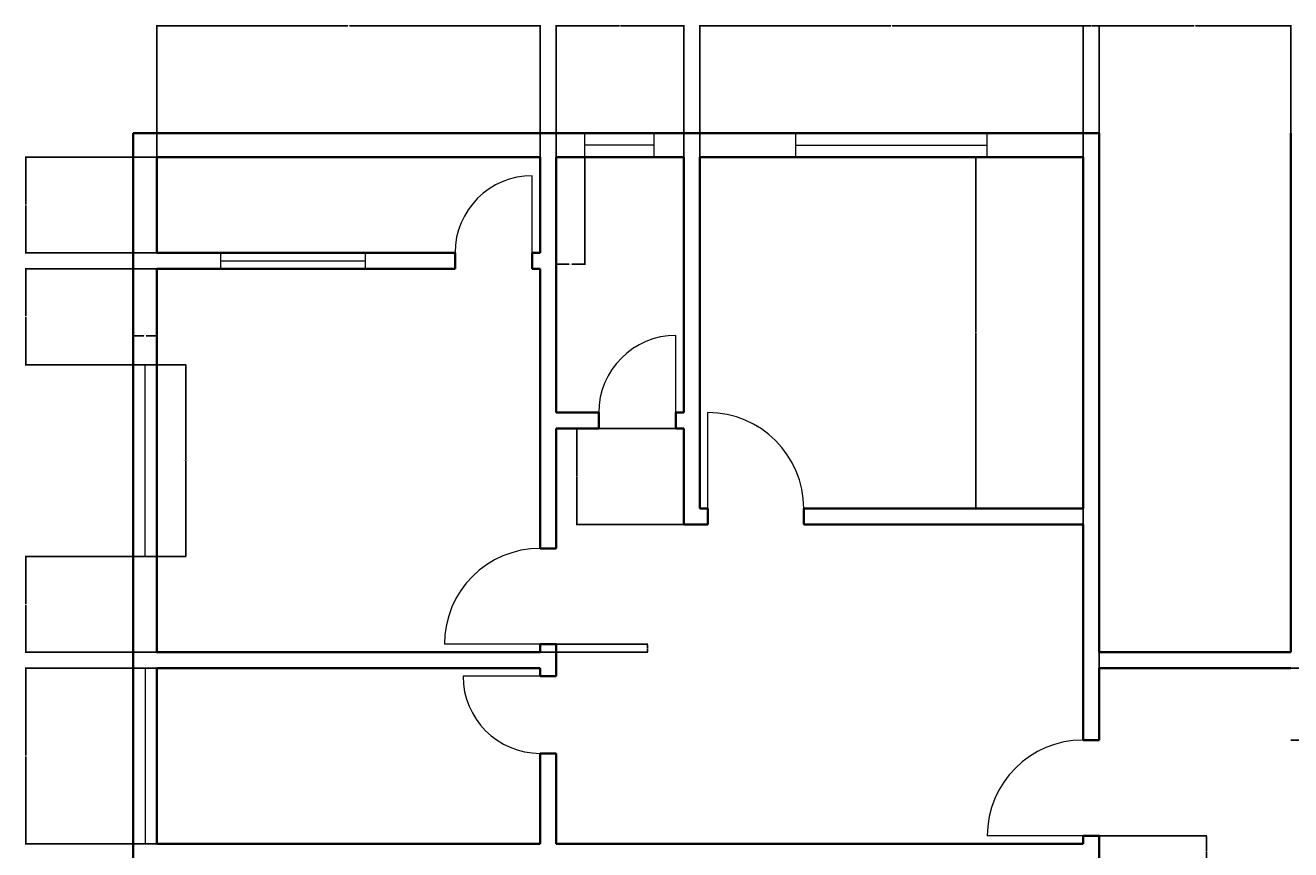
# Model space of a CAD drawing. Units: inches. Extents: x 2811 to 3694, y 2039 to 2670.
# Tile 2 of 3: x 2811 to 3286, y 2361 to 2670. Entities that reach past the tile are written whole.
import ezdxf

# ---------------------------------------------------------------- set-up
doc = ezdxf.new("R2010")
doc.units = ezdxf.units.IN
for name, color, linetype, lineweight in [('A-ANNO-DIMS', 2, 'Continuous', 18), ('A-DOOR', 3, 'Continuous', 18), ('A-GLAZ', 4, 'Continuous', 18), ('A-WALL', 7, 'Continuous', 35)]:
    doc.layers.add(name, color=color, linetype=linetype, lineweight=lineweight)
doc.styles.get("Standard").update_dxf_attribs({"font": 'arial.ttf'})
doc.dimstyles.get("Standard").update_dxf_attribs({"dimtxt": 0.18, "dimasz": 0.18, "dimexe": 0.18, "dimexo": 0.0625, "dimgap": 0.09, "dimtad": 0, "dimtih": 1, "dimtoh": 1, "dimdec": 4, "dimzin": 0, "dimdsep": 46, "dimtxsty": 'Standard', "dimcen": 0.09, "dimadec": 0, "dimazin": 0, "dimtfac": 1, "dimtdec": 4, "dimtofl": 0, "dimtmove": 0, "dimatfit": 3, "dimfxl": 1, "dimtolj": 1, "dimtzin": 0, "dimarcsym": 0})

# ---------------------------------------------------------------- blocks, each defined once
blk = doc.blocks.new('DOOR-SWING-29IN')
blk.add_line((29, 0), (29, 29))
blk.add_arc((29, 0), 29, 90, 180)
blk = doc.blocks.new('DOOR-SWING-36IN')
blk.add_line((36, 0), (0, 0))
blk.add_arc((36, 0), 36, 90, 180)
blk = doc.blocks.new('WIN-72IN')
for p, q in [((0, 0), (0, 9)), ((72, 0), (72, 9)), ((0, 4.5), (72, 4.5))]:
    blk.add_line(p, q)
blk = doc.blocks.new('WIN-66IN')
for p, q in [((0, 66), (9, 66)), ((4.5, 0), (4.5, 66)), ((0, 0), (9, 0))]:
    blk.add_line(p, q)
blk = doc.blocks.new('WIN-26_08IN')
for p, q in [((0, 0), (0, 9)), ((26.08, 0), (26.08, 9)), ((26.08, 4.5), (0, 4.5))]:
    blk.add_line(p, q)
blk = doc.blocks.new('*D14')
at = {"layer": 'A-ANNO-DIMS', "color": 0, "lineweight": -2, "transparency": 16777216}
for p, q in [((2860.34, 2542.98), (2871.26, 2542.98)), ((2871.08, 2542.8), (2871.08, 2507.16)), ((2871.08, 2471.16), (2871.08, 2506.8)), ((2860.34, 2470.98), (2871.26, 2470.98))]:
    blk.add_line(p, q, dxfattribs=at)
at = {"layer": 'A-ANNO-DIMS', "color": 0, "transparency": 16777216}
for points in [[(2871.05, 2542.8), (2871.11, 2542.8), (2871.08, 2542.98)], [(2871.05, 2471.16), (2871.11, 2471.16), (2871.08, 2470.98)]]:
    blk.add_solid(points, dxfattribs=at)
at = {"layer": 'Defpoints', "color": 0, "transparency": 16777216}
for p in [(2860.28, 2542.98), (2871.08, 2542.98), (2860.28, 2470.98)]:
    blk.add_point(p, dxfattribs=at)
at = {"layer": 'A-ANNO-DIMS', "color": 0, "transparency": 16777216, "insert": (2871.08, 2506.98), "char_height": 0.18, "attachment_point": 5}
blk.add_mtext('\\A1;WINDOW 72 TYP.', dxfattribs=at)
blk = doc.blocks.new('*D15')
at = {"layer": 'A-ANNO-DIMS', "color": 0, "lineweight": -2, "transparency": 16777216}
for p, q in [((2851.28, 2543.04), (2851.28, 2553.96)), ((2851.46, 2553.78), (2855.32, 2553.78)), ((2860.1, 2553.78), (2856.23, 2553.78)), ((2860.28, 2543.04), (2860.28, 2553.96))]:
    blk.add_line(p, q, dxfattribs=at)
at = {"layer": 'A-ANNO-DIMS', "color": 0, "transparency": 16777216}
for points in [[(2851.46, 2553.81), (2851.46, 2553.75), (2851.28, 2553.78)], [(2860.1, 2553.81), (2860.1, 2553.75), (2860.28, 2553.78)]]:
    blk.add_solid(points, dxfattribs=at)
at = {"layer": 'Defpoints', "color": 0, "transparency": 16777216}
for p in [(2851.28, 2553.78), (2851.28, 2542.98), (2860.28, 2542.98)]:
    blk.add_point(p, dxfattribs=at)
at = {"layer": 'A-ANNO-DIMS', "color": 0, "transparency": 16777216, "insert": (2855.78, 2553.78), "char_height": 0.18, "attachment_point": 5}
blk.add_mtext('\\A1;9 TYP.', dxfattribs=at)
blk = doc.blocks.new('*D24')
at = {"layer": 'A-ANNO-DIMS', "color": 0, "lineweight": -2, "transparency": 16777216}
for p, q in [((2860.28, 2621.04), (2860.28, 2670.46)), ((2860.46, 2670.28), (2932, 2670.28)), ((3004.1, 2670.28), (2932.56, 2670.28)), ((3004.28, 2621.04), (3004.28, 2670.46))]:
    blk.add_line(p, q, dxfattribs=at)
at = {"layer": 'A-ANNO-DIMS', "color": 0, "transparency": 16777216}
for points in [[(2860.46, 2670.31), (2860.46, 2670.25), (2860.28, 2670.28)], [(3004.1, 2670.31), (3004.1, 2670.25), (3004.28, 2670.28)]]:
    blk.add_solid(points, dxfattribs=at)
at = {"layer": 'Defpoints', "color": 0, "transparency": 16777216}
for p in [(3004.28, 2670.28), (2860.28, 2620.98), (3004.28, 2620.98)]:
    blk.add_point(p, dxfattribs=at)
at = {"layer": 'A-ANNO-DIMS', "color": 0, "transparency": 16777216, "insert": (2932.28, 2670.28), "char_height": 0.18, "attachment_point": 5}
blk.add_mtext('\\A1;144', dxfattribs=at)
blk = doc.blocks.new('*D25')
at = {"layer": 'A-ANNO-DIMS', "color": 0, "lineweight": -2, "transparency": 16777216}
for p, q in [((3010.28, 2621.04), (3010.28, 2670.46)), ((3010.46, 2670.28), (3034.05, 2670.28)), ((3058.1, 2670.28), (3034.5, 2670.28)), ((3058.28, 2621.04), (3058.28, 2670.46))]:
    blk.add_line(p, q, dxfattribs=at)
at = {"layer": 'A-ANNO-DIMS', "color": 0, "transparency": 16777216}
for points in [[(3010.46, 2670.31), (3010.46, 2670.25), (3010.28, 2670.28)], [(3058.1, 2670.31), (3058.1, 2670.25), (3058.28, 2670.28)]]:
    blk.add_solid(points, dxfattribs=at)
at = {"layer": 'Defpoints', "color": 0, "transparency": 16777216}
for p in [(3058.28, 2670.28), (3010.28, 2620.98), (3058.28, 2620.98)]:
    blk.add_point(p, dxfattribs=at)
at = {"layer": 'A-ANNO-DIMS', "color": 0, "transparency": 16777216, "insert": (3034.28, 2670.28), "char_height": 0.18, "attachment_point": 5}
blk.add_mtext('\\A1;48', dxfattribs=at)
blk = doc.blocks.new('*D26')
at = {"layer": 'A-ANNO-DIMS', "color": 0, "lineweight": -2, "transparency": 16777216}
for p, q in [((3064.28, 2621.04), (3064.28, 2670.46)), ((3064.46, 2670.28), (3136, 2670.28)), ((3208.1, 2670.28), (3136.56, 2670.28)), ((3208.28, 2621.04), (3208.28, 2670.46))]:
    blk.add_line(p, q, dxfattribs=at)
at = {"layer": 'A-ANNO-DIMS', "color": 0, "transparency": 16777216}
for points in [[(3064.46, 2670.31), (3064.46, 2670.25), (3064.28, 2670.28)], [(3208.1, 2670.31), (3208.1, 2670.25), (3208.28, 2670.28)]]:
    blk.add_solid(points, dxfattribs=at)
at = {"layer": 'Defpoints', "color": 0, "transparency": 16777216}
for p in [(3208.28, 2670.28), (3064.28, 2620.98), (3208.28, 2620.98)]:
    blk.add_point(p, dxfattribs=at)
at = {"layer": 'A-ANNO-DIMS', "color": 0, "transparency": 16777216, "insert": (3136.28, 2670.28), "char_height": 0.18, "attachment_point": 5}
blk.add_mtext('\\A1;144', dxfattribs=at)
blk = doc.blocks.new('*D27')
at = {"layer": 'A-ANNO-DIMS', "color": 0, "lineweight": -2, "transparency": 16777216}
for p, q in [((3214.28, 2630.04), (3214.28, 2670.46)), ((3214.46, 2670.28), (3250.06, 2670.28)), ((3286.1, 2670.28), (3250.49, 2670.28)), ((3286.28, 2630.04), (3286.28, 2670.46))]:
    blk.add_line(p, q, dxfattribs=at)
at = {"layer": 'A-ANNO-DIMS', "color": 0, "transparency": 16777216}
for points in [[(3214.46, 2670.31), (3214.46, 2670.25), (3214.28, 2670.28)], [(3286.1, 2670.31), (3286.1, 2670.25), (3286.28, 2670.28)]]:
    blk.add_solid(points, dxfattribs=at)
at = {"layer": 'Defpoints', "color": 0, "transparency": 16777216}
for p in [(3286.28, 2670.28), (3214.28, 2629.98), (3286.28, 2629.98)]:
    blk.add_point(p, dxfattribs=at)
at = {"layer": 'A-ANNO-DIMS', "color": 0, "transparency": 16777216, "insert": (3250.28, 2670.28), "char_height": 0.18, "attachment_point": 5}
blk.add_mtext('\\A1;72', dxfattribs=at)
blk = doc.blocks.new('*D31')
at = {"layer": 'A-ANNO-DIMS', "color": 0, "lineweight": -2, "transparency": 16777216}
for p, q in [((2860.21, 2620.98), (2810.8, 2620.98)), ((2810.98, 2620.8), (2810.98, 2603.16)), ((2810.98, 2585.16), (2810.98, 2602.8)), ((2860.21, 2584.98), (2810.8, 2584.98))]:
    blk.add_line(p, q, dxfattribs=at)
at = {"layer": 'A-ANNO-DIMS', "color": 0, "transparency": 16777216}
for points in [[(2810.95, 2620.8), (2811.01, 2620.8), (2810.98, 2620.98)], [(2810.95, 2585.16), (2811.01, 2585.16), (2810.98, 2584.98)]]:
    blk.add_solid(points, dxfattribs=at)
at = {"layer": 'Defpoints', "color": 0, "transparency": 16777216}
for p in [(2860.28, 2620.98), (2810.98, 2584.98), (2860.28, 2584.98)]:
    blk.add_point(p, dxfattribs=at)
at = {"layer": 'A-ANNO-DIMS', "color": 0, "transparency": 16777216, "insert": (2810.98, 2602.98), "char_height": 0.18, "attachment_point": 5}
blk.add_mtext('\\A1;36', dxfattribs=at)
blk = doc.blocks.new('*D32')
at = {"layer": 'A-ANNO-DIMS', "color": 0, "lineweight": -2, "transparency": 16777216}
for p, q in [((2860.21, 2578.98), (2810.8, 2578.98)), ((2810.98, 2578.8), (2810.98, 2561.16)), ((2810.98, 2543.16), (2810.98, 2560.8)), ((2860.21, 2542.98), (2810.8, 2542.98))]:
    blk.add_line(p, q, dxfattribs=at)
at = {"layer": 'A-ANNO-DIMS', "color": 0, "transparency": 16777216}
for points in [[(2810.95, 2578.8), (2811.01, 2578.8), (2810.98, 2578.98)], [(2810.95, 2543.16), (2811.01, 2543.16), (2810.98, 2542.98)]]:
    blk.add_solid(points, dxfattribs=at)
at = {"layer": 'Defpoints', "color": 0, "transparency": 16777216}
for p in [(2860.28, 2578.98), (2810.98, 2542.98), (2860.28, 2542.98)]:
    blk.add_point(p, dxfattribs=at)
at = {"layer": 'A-ANNO-DIMS', "color": 0, "transparency": 16777216, "insert": (2810.98, 2560.98), "char_height": 0.18, "attachment_point": 5}
blk.add_mtext('\\A1;36', dxfattribs=at)
blk = doc.blocks.new('*D33')
at = {"layer": 'A-ANNO-DIMS', "color": 0, "lineweight": -2, "transparency": 16777216}
for p, q in [((2860.21, 2470.98), (2810.8, 2470.98)), ((2810.98, 2470.8), (2810.98, 2453.16)), ((2810.98, 2435.16), (2810.98, 2452.8)), ((2860.21, 2434.98), (2810.8, 2434.98))]:
    blk.add_line(p, q, dxfattribs=at)
at = {"layer": 'A-ANNO-DIMS', "color": 0, "transparency": 16777216}
for points in [[(2810.95, 2470.8), (2811.01, 2470.8), (2810.98, 2470.98)], [(2810.95, 2435.16), (2811.01, 2435.16), (2810.98, 2434.98)]]:
    blk.add_solid(points, dxfattribs=at)
at = {"layer": 'Defpoints', "color": 0, "transparency": 16777216}
for p in [(2860.28, 2470.98), (2810.98, 2434.98), (2860.28, 2434.98)]:
    blk.add_point(p, dxfattribs=at)
at = {"layer": 'A-ANNO-DIMS', "color": 0, "transparency": 16777216, "insert": (2810.98, 2452.98), "char_height": 0.18, "attachment_point": 5}
blk.add_mtext('\\A1;36', dxfattribs=at)
blk = doc.blocks.new('*D34')
at = {"layer": 'A-ANNO-DIMS', "color": 0, "lineweight": -2, "transparency": 16777216}
for p, q in [((2860.21, 2428.98), (2810.8, 2428.98)), ((2810.98, 2428.8), (2810.98, 2396.16)), ((2810.98, 2363.16), (2810.98, 2395.8)), ((2860.21, 2362.98), (2810.8, 2362.98))]:
    blk.add_line(p, q, dxfattribs=at)
at = {"layer": 'A-ANNO-DIMS', "color": 0, "transparency": 16777216}
for points in [[(2810.95, 2428.8), (2811.01, 2428.8), (2810.98, 2428.98)], [(2810.95, 2363.16), (2811.01, 2363.16), (2810.98, 2362.98)]]:
    blk.add_solid(points, dxfattribs=at)
at = {"layer": 'Defpoints', "color": 0, "transparency": 16777216}
for p in [(2860.28, 2428.98), (2810.98, 2362.98), (2860.28, 2362.98)]:
    blk.add_point(p, dxfattribs=at)
at = {"layer": 'A-ANNO-DIMS', "color": 0, "transparency": 16777216, "insert": (2810.98, 2395.98), "char_height": 0.18, "attachment_point": 5}
blk.add_mtext('\\A1;66', dxfattribs=at)
blk = doc.blocks.new('*D40')
at = {"layer": 'A-ANNO-DIMS', "color": 0, "lineweight": -2, "transparency": 16777216}
for p, q in [((3058.21, 2518.98), (3017.8, 2518.98)), ((3017.98, 2518.8), (3017.98, 2501.16)), ((3017.98, 2483.16), (3017.98, 2500.8)), ((3058.21, 2482.98), (3017.8, 2482.98))]:
    blk.add_line(p, q, dxfattribs=at)
at = {"layer": 'A-ANNO-DIMS', "color": 0, "transparency": 16777216}
for points in [[(3017.95, 2518.8), (3018.01, 2518.8), (3017.98, 2518.98)], [(3017.95, 2483.16), (3018.01, 2483.16), (3017.98, 2482.98)]]:
    blk.add_solid(points, dxfattribs=at)
at = {"layer": 'Defpoints', "color": 0, "transparency": 16777216}
for p in [(3017.98, 2518.98), (3058.28, 2518.98), (3058.28, 2482.98)]:
    blk.add_point(p, dxfattribs=at)
at = {"layer": 'A-ANNO-DIMS', "color": 0, "transparency": 16777216, "insert": (3017.98, 2500.98), "char_height": 0.18, "attachment_point": 5}
blk.add_mtext('\\A1;36', dxfattribs=at)
blk = doc.blocks.new('*D41')
at = {"layer": 'A-ANNO-DIMS', "color": 0, "lineweight": -2, "transparency": 16777216}
for p, q in [((3208.21, 2620.98), (3167.8, 2620.98)), ((3167.98, 2620.8), (3167.98, 2555.16)), ((3167.98, 2489.16), (3167.98, 2554.8)), ((3208.21, 2488.98), (3167.8, 2488.98))]:
    blk.add_line(p, q, dxfattribs=at)
at = {"layer": 'A-ANNO-DIMS', "color": 0, "transparency": 16777216}
for points in [[(3167.95, 2620.8), (3168.01, 2620.8), (3167.98, 2620.98)], [(3167.95, 2489.16), (3168.01, 2489.16), (3167.98, 2488.98)]]:
    blk.add_solid(points, dxfattribs=at)
at = {"layer": 'Defpoints', "color": 0, "transparency": 16777216}
for p in [(3167.98, 2620.98), (3208.28, 2620.98), (3208.28, 2488.98)]:
    blk.add_point(p, dxfattribs=at)
at = {"layer": 'A-ANNO-DIMS', "color": 0, "transparency": 16777216, "insert": (3167.98, 2554.98), "char_height": 0.18, "attachment_point": 5}
blk.add_mtext('\\A1;132', dxfattribs=at)
blk = doc.blocks.new('*D52')
at = {"layer": 'A-ANNO-DIMS', "color": 0, "lineweight": -2, "transparency": 16777216}
for p, q in [((3010.28, 2620.92), (3010.28, 2580.5)), ((3021.03, 2620.92), (3021.03, 2580.5)), ((3010.46, 2580.68), (3015.2, 2580.68)), ((3020.85, 2580.68), (3016.11, 2580.68))]:
    blk.add_line(p, q, dxfattribs=at)
at = {"layer": 'A-ANNO-DIMS', "color": 0, "transparency": 16777216}
for points in [[(3010.46, 2580.71), (3010.46, 2580.65), (3010.28, 2580.68)], [(3020.85, 2580.71), (3020.85, 2580.65), (3021.03, 2580.68)]]:
    blk.add_solid(points, dxfattribs=at)
at = {"layer": 'Defpoints', "color": 0, "transparency": 16777216}
for p in [(3010.28, 2620.98), (3021.03, 2620.98), (3010.28, 2580.68)]:
    blk.add_point(p, dxfattribs=at)
at = {"layer": 'A-ANNO-DIMS', "color": 0, "transparency": 16777216, "insert": (3015.65, 2580.68), "char_height": 0.18, "attachment_point": 5}
blk.add_mtext('\\A1;10.754', dxfattribs=at)
blk = doc.blocks.new('*D54')
at = {"layer": 'A-ANNO-DIMS', "color": 0, "lineweight": -2, "transparency": 16777216}
for p, q in [((3004.34, 2437.98), (3044.76, 2437.98)), ((3004.34, 2434.98), (3044.76, 2434.98)), ((3044.58, 2437.8), (3044.58, 2436.66)), ((3044.58, 2435.16), (3044.58, 2436.3))]:
    blk.add_line(p, q, dxfattribs=at)
at = {"layer": 'A-ANNO-DIMS', "color": 0, "transparency": 16777216}
for points in [[(3044.55, 2437.8), (3044.61, 2437.8), (3044.58, 2437.98)], [(3044.55, 2435.16), (3044.61, 2435.16), (3044.58, 2434.98)]]:
    blk.add_solid(points, dxfattribs=at)
at = {"layer": 'Defpoints', "color": 0, "transparency": 16777216}
for p in [(3004.28, 2437.98), (3004.28, 2434.98), (3044.58, 2434.98)]:
    blk.add_point(p, dxfattribs=at)
at = {"layer": 'A-ANNO-DIMS', "color": 0, "transparency": 16777216, "insert": (3044.58, 2436.48), "char_height": 0.18, "attachment_point": 5}
blk.add_mtext('\\A1;3', dxfattribs=at)
blk = doc.blocks.new('*D60')
at = {"layer": 'A-ANNO-DIMS', "color": 0, "lineweight": -2, "transparency": 16777216}
for p, q in [((3286.34, 2428.98), (3326.76, 2428.98)), ((3326.58, 2428.8), (3326.58, 2415.66)), ((3326.58, 2402.16), (3326.58, 2415.3)), ((3286.34, 2401.98), (3326.76, 2401.98))]:
    blk.add_line(p, q, dxfattribs=at)
at = {"layer": 'A-ANNO-DIMS', "color": 0, "transparency": 16777216}
for points in [[(3326.55, 2428.8), (3326.61, 2428.8), (3326.58, 2428.98)], [(3326.55, 2402.16), (3326.61, 2402.16), (3326.58, 2401.98)]]:
    blk.add_solid(points, dxfattribs=at)
at = {"layer": 'Defpoints', "color": 0, "transparency": 16777216}
for p in [(3286.28, 2428.98), (3286.28, 2401.98), (3326.58, 2401.98)]:
    blk.add_point(p, dxfattribs=at)
at = {"layer": 'A-ANNO-DIMS', "color": 0, "transparency": 16777216, "insert": (3326.58, 2415.48), "char_height": 0.18, "attachment_point": 5}
blk.add_mtext('\\A1;27', dxfattribs=at)
blk = doc.blocks.new('*D61')
at = {"layer": 'A-ANNO-DIMS', "color": 0, "lineweight": -2, "transparency": 16777216}
for p, q in [((3208.28, 2402.04), (3208.28, 2670.46)), ((3208.46, 2670.28), (3211.13, 2670.28)), ((3214.1, 2670.28), (3211.43, 2670.28)), ((3214.28, 2402.04), (3214.28, 2670.46))]:
    blk.add_line(p, q, dxfattribs=at)
at = {"layer": 'A-ANNO-DIMS', "color": 0, "transparency": 16777216}
for points in [[(3208.46, 2670.31), (3208.46, 2670.25), (3208.28, 2670.28)], [(3214.1, 2670.31), (3214.1, 2670.25), (3214.28, 2670.28)]]:
    blk.add_solid(points, dxfattribs=at)
at = {"layer": 'Defpoints', "color": 0, "transparency": 16777216}
for p in [(3214.28, 2670.28), (3208.28, 2401.98), (3214.28, 2401.98)]:
    blk.add_point(p, dxfattribs=at)
at = {"layer": 'A-ANNO-DIMS', "color": 0, "transparency": 16777216, "insert": (3211.28, 2670.28), "char_height": 0.18, "attachment_point": 5}
blk.add_mtext('\\A1;6', dxfattribs=at)
blk = doc.blocks.new('*D62')
at = {"layer": 'A-ANNO-DIMS', "color": 0, "lineweight": -2, "transparency": 16777216}
for p, q in [((3214.34, 2365.98), (3254.76, 2365.98)), ((3254.58, 2365.8), (3254.58, 2360.16)), ((3254.58, 2354.16), (3254.58, 2359.8)), ((3214.34, 2353.98), (3254.76, 2353.98))]:
    blk.add_line(p, q, dxfattribs=at)
at = {"layer": 'A-ANNO-DIMS', "color": 0, "transparency": 16777216}
for points in [[(3254.55, 2365.8), (3254.61, 2365.8), (3254.58, 2365.98)], [(3254.55, 2354.16), (3254.61, 2354.16), (3254.58, 2353.98)]]:
    blk.add_solid(points, dxfattribs=at)
at = {"layer": 'Defpoints', "color": 0, "transparency": 16777216}
for p in [(3214.28, 2365.98), (3214.28, 2353.98), (3254.58, 2353.98)]:
    blk.add_point(p, dxfattribs=at)
at = {"layer": 'A-ANNO-DIMS', "color": 0, "transparency": 16777216, "insert": (3254.58, 2359.98), "char_height": 0.18, "attachment_point": 5}
blk.add_mtext('\\A1;12', dxfattribs=at)

msp = doc.modelspace()

# ---------------------------------------------------------------- linework, layer by layer
at = {"layer": 'A-GLAZ'}
for p, q in [((3100.2765, 2625.4792), (3172.2765, 2625.4792)), ((2884.2647, 2578.9792), (2884.2647, 2584.9792)), ((2884.2647, 2581.9792), (2938.6787, 2581.9792)), ((2884.2647, 2581.9792), (2938.6787, 2581.9792)), ((2938.6787, 2578.9792), (2938.6787, 2584.9792)), ((2851.2765, 2470.9792), (2851.2765, 2542.9792)), ((2860.2765, 2542.9792), (2855.7765, 2542.9792)), ((2851.2765, 2362.9792), (2851.2765, 2428.9792)), ((2860.2765, 2428.9792), (2855.7765, 2428.9792))]:
    msp.add_line(p, q, dxfattribs=at)
at = {"layer": 'A-WALL'}
for p, q in [((2851.2765, 2629.9792), (2851.2765, 2124.9792)), ((3214.2765, 2629.9792), (2851.2765, 2629.9792)), ((3214.2765, 2620.9792), (3214.2765, 2629.9792)), ((3286.2765, 2620.9792), (3286.2765, 2629.9792)), ((2860.2765, 2620.9792), (2860.2765, 2584.9792)), ((3004.2765, 2620.9792), (2860.2765, 2620.9792)), ((3004.2765, 2620.9792), (3004.2765, 2584.9792)), ((3010.2765, 2620.9792), (3010.2765, 2524.9792)), ((3058.2765, 2620.9792), (3010.2765, 2620.9792)), ((3058.2765, 2620.9792), (3058.2765, 2524.9792)), ((3064.2765, 2620.9792), (3064.2765, 2488.9792)), ((3208.2765, 2620.9792), (3064.2765, 2620.9792)), ((3208.2765, 2620.9792), (3208.2765, 2488.9792)), ((3214.2765, 2620.9792), (3214.2765, 2434.9792)), ((3286.2765, 2620.9792), (3286.2765, 2434.9792)), ((2972.2765, 2584.9792), (2860.2765, 2584.9792)), ((2972.2765, 2584.9792), (2972.2765, 2578.9792)), ((3004.2765, 2584.9792), (3001.2765, 2584.9792)), ((3001.2765, 2584.9792), (3001.2765, 2578.9792)), ((2860.2765, 2578.9792), (2860.2765, 2434.9792)), ((2972.2765, 2578.9792), (2860.2765, 2578.9792)), ((3004.2765, 2578.9792), (3001.2765, 2578.9792)), ((3004.2765, 2578.9792), (3004.2765, 2473.9792)), ((3026.2765, 2524.9792), (3010.2765, 2524.9792)), ((3026.2765, 2524.9792), (3026.2765, 2518.9792)), ((3058.2765, 2524.9792), (3055.2765, 2524.9792)), ((3055.2765, 2524.9792), (3055.2765, 2518.9792)), ((3010.2765, 2518.9792), (3010.2765, 2473.9792)), ((3026.2765, 2518.9792), (3010.2765, 2518.9792)), ((3058.2765, 2518.9792), (3055.2765, 2518.9792)), ((3058.2765, 2518.9792), (3058.2765, 2482.9792)), ((3067.2765, 2488.9792), (3064.2765, 2488.9792)), ((3067.2765, 2488.9792), (3067.2765, 2482.9792)), ((3208.2765, 2488.9792), (3103.2765, 2488.9792)), ((3103.2765, 2488.9792), (3103.2765, 2482.9792)), ((3064.2765, 2482.9792), (3058.2765, 2482.9792)), ((3067.2765, 2482.9792), (3064.2765, 2482.9792)), ((3208.2765, 2482.9792), (3103.2765, 2482.9792)), ((3208.2765, 2482.9792), (3208.2765, 2401.9792)), ((3004.2765, 2473.9792), (3010.2765, 2473.9792)), ((3004.2765, 2434.9792), (2860.2765, 2434.9792)), ((3004.2765, 2437.9792), (3010.2765, 2437.9792)), ((3004.2765, 2437.9792), (3004.2765, 2434.9792)), ((3010.2765, 2437.9792), (3010.2765, 2425.9792)), ((3214.2765, 2434.9792), (3286.2765, 2434.9792)), ((3004.2765, 2428.9792), (2860.2765, 2428.9792)), ((2860.2765, 2428.9792), (2860.2765, 2362.9792)), ((3004.2765, 2428.9792), (3004.2765, 2425.9792)), ((3004.2765, 2425.9792), (3010.2765, 2425.9792)), ((3286.2765, 2428.9792), (3214.2765, 2428.9792)), ((3214.2765, 2428.9792), (3214.2765, 2401.9792)), ((3208.2765, 2401.9792), (3214.2765, 2401.9792)), ((3004.2765, 2396.9792), (3010.2765, 2396.9792)), ((3004.2765, 2396.9792), (3004.2765, 2362.9792)), ((3010.2765, 2396.9792), (3010.2765, 2362.9792)), ((3208.2765, 2365.9792), (3214.2765, 2365.9792)), ((3208.2765, 2365.9792), (3208.2765, 2362.9792)), ((3214.2765, 2365.9792), (3214.2765, 2353.9792)), ((3004.2765, 2362.9792), (2860.2765, 2362.9792)), ((3208.2765, 2362.9792), (3010.2765, 2362.9792))]:
    msp.add_line(p, q, dxfattribs=at)

# ---------------------------------------------------------------- block references
at = {"layer": 'A-DOOR'}
for name, p in [('DOOR-SWING-29IN', (2972.277, 2584.979)), ('DOOR-SWING-29IN', (3026.277, 2524.979)), ('DOOR-SWING-36IN', (2968.277, 2437.979)), ('DOOR-SWING-36IN', (3172.277, 2365.979))]:
    msp.add_blockref(name, p, dxfattribs=at)
for name, p, rotation in [('DOOR-SWING-36IN', (3067.2763, 2524.9788), 270), ('DOOR-SWING-29IN', (3004.2768, 2396.9797), 90)]:
    msp.add_blockref(name, p, dxfattribs=dict(at, rotation=rotation))
at = {"layer": 'A-GLAZ'}
for name, p in [('WIN-26_08IN', (3021.031, 2620.979)), ('WIN-72IN', (3100.277, 2620.979))]:
    msp.add_blockref(name, p, dxfattribs=at)
for name, p, rotation in [('WIN-72IN', (2860.2768, 2470.9797), 89.9999999999986), ('WIN-66IN', (2860.2761, 2428.9795), 180)]:
    msp.add_blockref(name, p, dxfattribs=dict(at, rotation=rotation))

# ---------------------------------------------------------------- dimensions: what is measured, and where the dimension line sits
at = {"layer": 'A-ANNO-DIMS'}
for base, p1, p2, picture, middle in [((3004.2765, 2670.2792), (2860.2765, 2620.9792), (3004.2765, 2620.9792), '*D24', (2932.2765, 2670.2792)), ((3058.2765, 2670.2792), (3010.2765, 2620.9792), (3058.2765, 2620.9792), '*D25', (3034.2765, 2670.2792)), ((3208.2765, 2670.2792), (3064.2765, 2620.9792), (3208.2765, 2620.9792), '*D26', (3136.2765, 2670.2792)), ((3214.2765, 2670.2792), (3208.2765, 2401.9792), (3214.2765, 2401.9792), '*D61', (3211.2765, 2670.2792)), ((3286.2765, 2670.2792), (3214.2765, 2629.9792), (3286.2765, 2629.9792), '*D27', (3250.2765, 2670.2792))]:
    dim = msp.add_linear_dim(base=base, p1=p1, p2=p2, dimstyle='Standard', override={"dimdec": 0, "dimlfac": 1, "dimrnd": 0, "dimzin": 0, "dimdsep": 46, "dimlunit": 2}, dxfattribs=at)
    dim.commit()
    dim.dimension.update_dxf_attribs({"geometry": picture, "text_midpoint": middle})
for base, p1, p2, angle, override, picture, middle in [((2810.9765, 2584.9792), (2860.2765, 2620.9792), (2860.2765, 2584.9792), 90, {"dimdec": 0, "dimlfac": 1, "dimrnd": 0, "dimzin": 0, "dimdsep": 46, "dimlunit": 2}, '*D31', (2810.9765, 2602.9792)), ((3010.2765, 2580.6792), (3021.0309, 2620.9792), (3010.2765, 2620.9792), 180, {"dimdec": 3, "dimlfac": 1, "dimrnd": 0, "dimzin": 0, "dimdsep": 46, "dimlunit": 2}, '*D52', (3015.6537, 2580.6792)), ((3167.9765, 2620.9792), (3208.2765, 2488.9792), (3208.2765, 2620.9792), 90, {"dimdec": 0, "dimlfac": 1, "dimrnd": 0, "dimzin": 0, "dimdsep": 46, "dimlunit": 2}, '*D41', (3167.9765, 2554.9792)), ((2810.9765, 2542.9792), (2860.2765, 2578.9792), (2860.2765, 2542.9792), 90, {"dimdec": 0, "dimlfac": 1, "dimrnd": 0, "dimzin": 0, "dimdsep": 46, "dimlunit": 2}, '*D32', (2810.9765, 2560.9792)), ((3017.9765, 2518.9792), (3058.2765, 2482.9792), (3058.2765, 2518.9792), 90, {"dimdec": 0, "dimlfac": 1, "dimrnd": 0, "dimzin": 0, "dimdsep": 46, "dimlunit": 2}, '*D40', (3017.9765, 2500.9792)), ((2810.9765, 2434.9792), (2860.2765, 2470.9792), (2860.2765, 2434.9792), 90, {"dimdec": 0, "dimlfac": 1, "dimrnd": 0, "dimzin": 0, "dimdsep": 46, "dimlunit": 2}, '*D33', (2810.9765, 2452.9792)), ((3044.5765, 2434.9792), (3004.2765, 2437.9792), (3004.2765, 2434.9792), 270, {"dimdec": 0, "dimlfac": 1, "dimrnd": 0, "dimzin": 0, "dimdsep": 46, "dimlunit": 2}, '*D54', (3044.5765, 2436.4792)), ((2810.9765, 2362.9792), (2860.2765, 2428.9792), (2860.2765, 2362.9792), 90, {"dimdec": 0, "dimlfac": 1, "dimrnd": 0, "dimzin": 0, "dimdsep": 46, "dimlunit": 2}, '*D34', (2810.9765, 2395.9792)), ((3326.5765, 2401.9792), (3286.2765, 2428.9792), (3286.2765, 2401.9792), 270, {"dimdec": 0, "dimlfac": 1, "dimrnd": 0, "dimzin": 0, "dimdsep": 46, "dimlunit": 2}, '*D60', (3326.5765, 2415.4792)), ((3254.5765, 2353.9792), (3214.2765, 2365.9792), (3214.2765, 2353.9792), 270, {"dimdec": 0, "dimlfac": 1, "dimrnd": 0, "dimzin": 0, "dimdsep": 46, "dimlunit": 2}, '*D62', (3254.5765, 2359.9792))]:
    dim = msp.add_linear_dim(base=base, p1=p1, p2=p2, angle=angle, dimstyle='Standard', override=override, dxfattribs=at)
    dim.commit()
    dim.dimension.update_dxf_attribs({"geometry": picture, "text_midpoint": middle})
for base, p1, p2, angle, text, picture, middle in [((2851.2765, 2553.7792), (2860.2765, 2542.9792), (2851.2765, 2542.9792), 180, '<> TYP.', '*D15', (2855.7765, 2553.7792)), ((2871.0765, 2542.9792), (2860.2765, 2470.9792), (2860.2765, 2542.9792), 90, 'WINDOW <> TYP.', '*D14', (2871.0765, 2506.9792))]:
    dim = msp.add_linear_dim(base=base, p1=p1, p2=p2, angle=angle, text=text, dimstyle='Standard', override={"dimdec": 0, "dimlfac": 1, "dimrnd": 0, "dimzin": 0, "dimdsep": 46, "dimlunit": 2}, dxfattribs=at)
    dim.commit()
    dim.dimension.update_dxf_attribs({"geometry": picture, "text_midpoint": middle})

doc.saveas('drawing.dxf')
